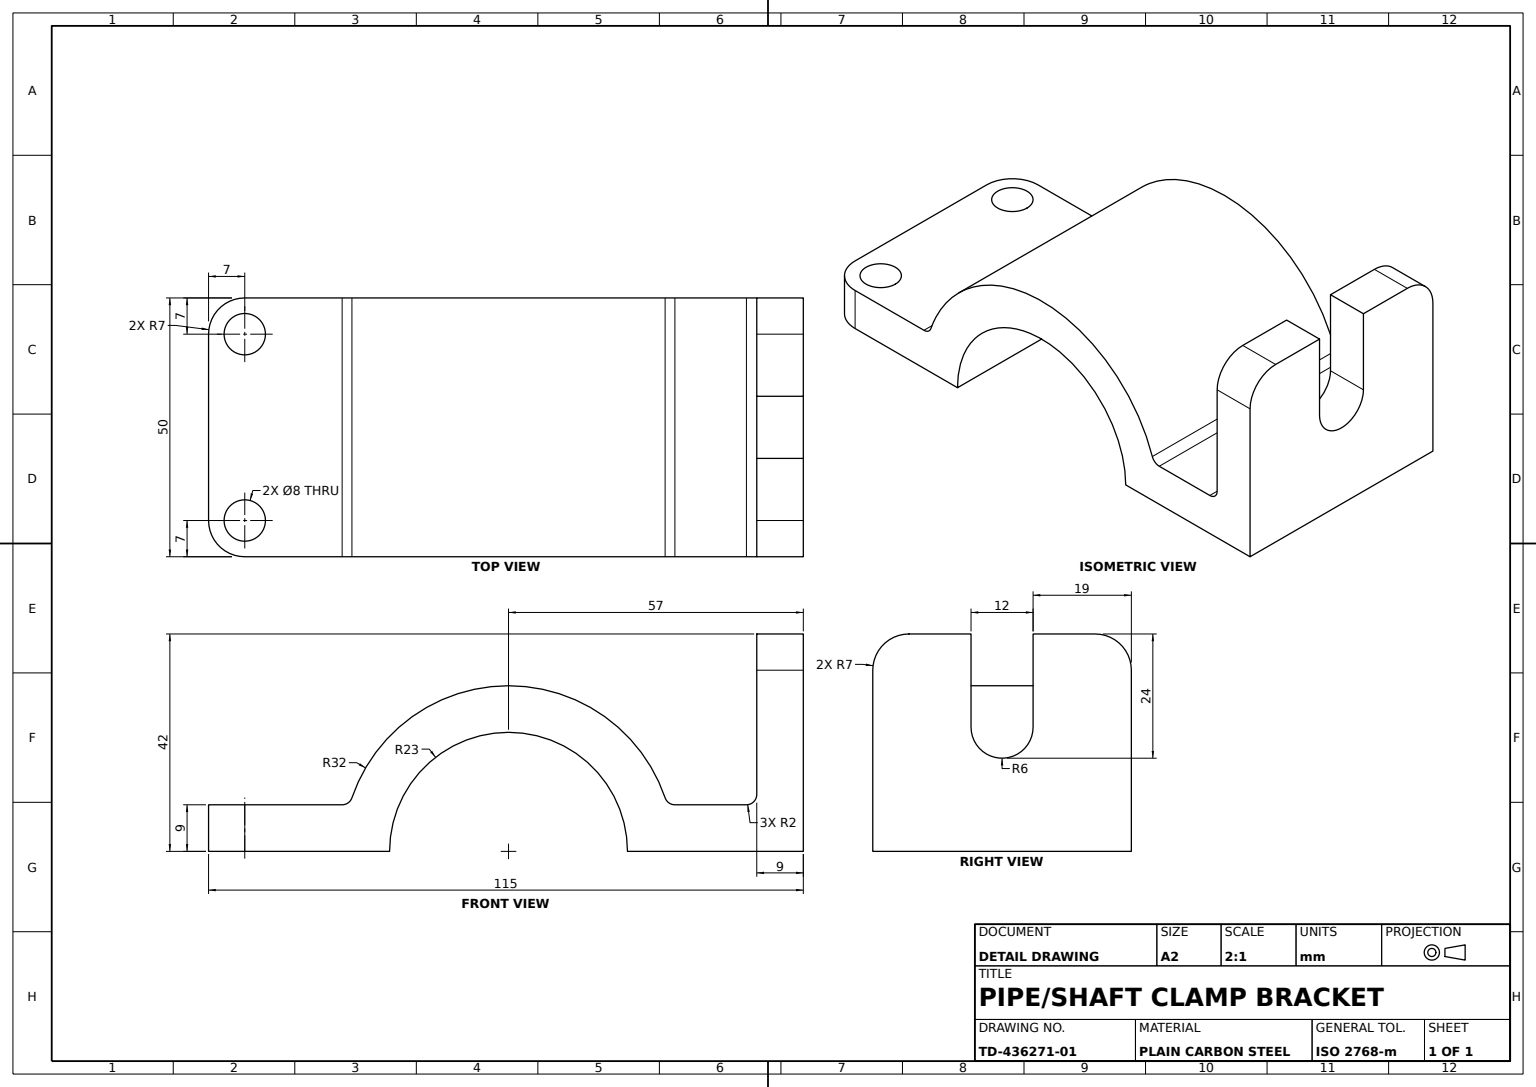
from build123d import *

# Parameters (mm, degrees)
SADDLE_BODY_DEPTH     = 25
EDGE_FILLETS_R2_R     = 2
CORNER_FILLETS_R7_R   = 7
FLANGE_HOLES_SKETCH_R = 4
FLANGE_HOLES_DEPTH    = 50
U_SLOT_CUT_DEPTH      = 20


with BuildPart() as part:
    # Saddle Profile Sketch → Saddle Body (new, symmetric)
    with BuildSketch(Plane.XY):
        with BuildLine():
            Line((-58, 0), (-23, 0))
            ThreePointArc((-23, 0), (0, 23), (23, 0))
            Line((23, 0), (57, 0))
            Line((57, 0), (57, 42))
            Line((57, 42), (48, 42))
            Line((48, 42), (48, 9))
            Line((48, 9), (30.708305066, 9))
            ThreePointArc((30.708305066, 9), (0, 32), (-30.708305066, 9))
            Line((-30.708305066, 9), (-58, 9))
            Line((-58, 9), (-58, 0))
        make_face()
    extrude(amount=SADDLE_BODY_DEPTH, both=True)

    # Edge Fillets R2
    edge_fillets_r2_edges = [part.edges().sort_by_distance(p)[0] for p in [
        (-30.708305066, 9, 0),
        (30.708305066, 9, 0),
        (48, 9, 0),
    ]]
    fillet(edge_fillets_r2_edges, radius=EDGE_FILLETS_R2_R)

    # Corner Fillets R7
    corner_fillets_r7_edges = [part.edges().sort_by_distance(p)[0] for p in [
        (-58, 4.5, -25),
        (52.5, 42, -25),
        (52.5, 42, 25),
        (-58, 4.5, 25),
    ]]
    fillet(corner_fillets_r7_edges, radius=CORNER_FILLETS_R7_R)

    # Flange Holes Sketch → Flange Holes (cut)
    with BuildSketch(Plane(origin=(0, 9, 0), x_dir=(1, 0, 0), z_dir=(0, 1, 0))):
        with Locations(Location((-51, 18, 0), (0, 0, 180))):
            Circle(FLANGE_HOLES_SKETCH_R)
        with Locations(Location((-51, -18, 0), (0, 0, 180))):
            Circle(FLANGE_HOLES_SKETCH_R)
    extrude(amount=-FLANGE_HOLES_DEPTH, mode=Mode.SUBTRACT)

    # U-Slot Sketch → U-Slot Cut (cut)
    with BuildSketch(Plane(origin=(57, 0, 0), x_dir=(0, 0, -1), z_dir=(1, 0, 0))):
        with BuildLine():
            Line((-6, 24), (-6, 44.935144294))
            ThreePointArc((-6, 44.935144294), (0, 50.935144294), (6, 44.935144294))
            Line((6, 44.935144294), (6, 24))
            ThreePointArc((6, 24), (0, 18), (-6, 24))
        make_face()
    extrude(amount=-U_SLOT_CUT_DEPTH, mode=Mode.SUBTRACT)


solid = part.part
